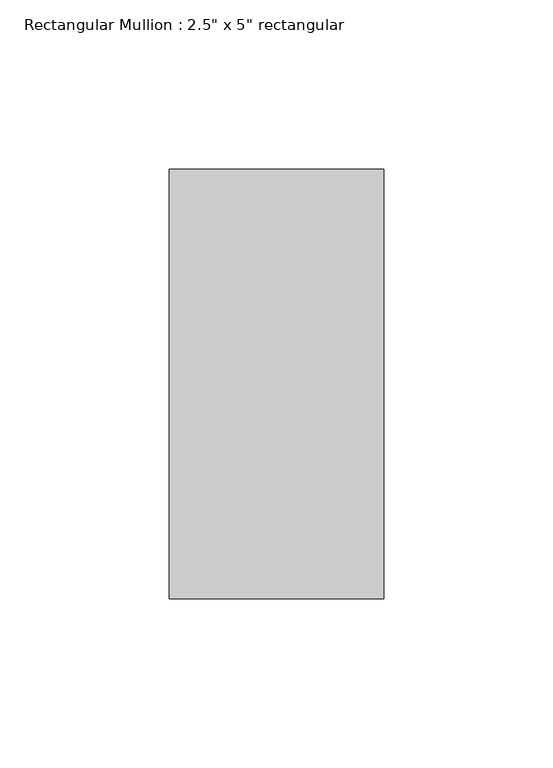
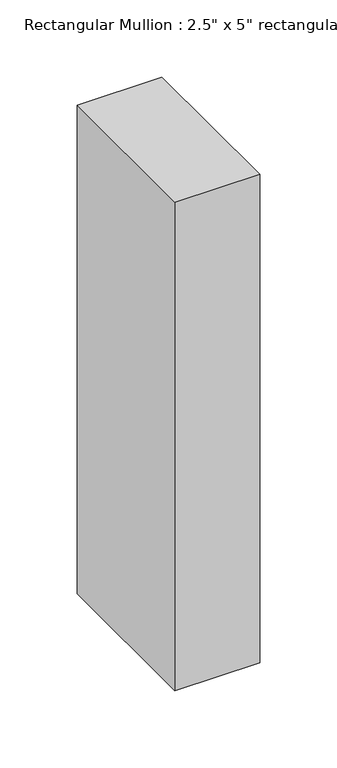
"""IFC4 building model written with IfcOpenShell, lengths in millimetres: member geometry."""

from ifc_helpers import new_model, si_unit, frame, origin, place, context, project, spatial, polyline, outline, extrude, source, transform, mapped, element, save


def member_dffdf235(model_context):
    return source(origin(), model_context, "Body", "SweptSolid", [
        extrude(outline(polyline([(0.0, 63.5), (0.0, -63.5), (-63.5, -63.5), (-63.5, 63.5), (0.0, 63.5)])), frame((0.0, 0.0, -387.35), z_axis=(0.0, 0.0, 1.0), x_axis=(1.0, 0.0, 0.0)), (0.0, 0.0, 1.0), 387.35),
    ])


if __name__ == "__main__":
    model = new_model("IFC4")
    model_context = context("Model", 3, world=origin())
    ifc_project = project(units=[si_unit("LENGTHUNIT", "METRE", prefix="MILLI")], contexts=[model_context])
    site = spatial("IfcSite", under=ifc_project)
    building = spatial("IfcBuilding", under=site)
    placement = place(None, origin())
    member_shape = member_dffdf235(model_context)
    element("IfcMember", 1, ObjectType="Rectangular Mullion : 2.5\" x 5\" rectangular", at=placement, inside=building, context=model_context, shape_type="MappedRepresentation", body=[
        mapped(member_shape, transform((0.0, 0.0, 0.0), x_axis=(1.0, 0.0, 0.0), y_axis=(0.0, 1.0, 0.0), z_axis=(0.0, 0.0, 1.0))),
    ])
    save(model, "model.ifc")

# Revit data of these elements
# Type "Rectangular Mullion : 2.5\" x 5\" rectangular"
#   built-in parameter 1007304 = 0.416667 (stored number, unit not read)
#   built-in parameter 1007301 = 0.104167 (stored number, unit not read)
#   built-in parameter 1007300 = 0.104167 (stored number, unit not read)
